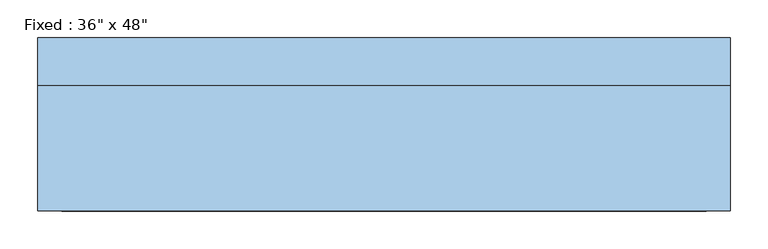
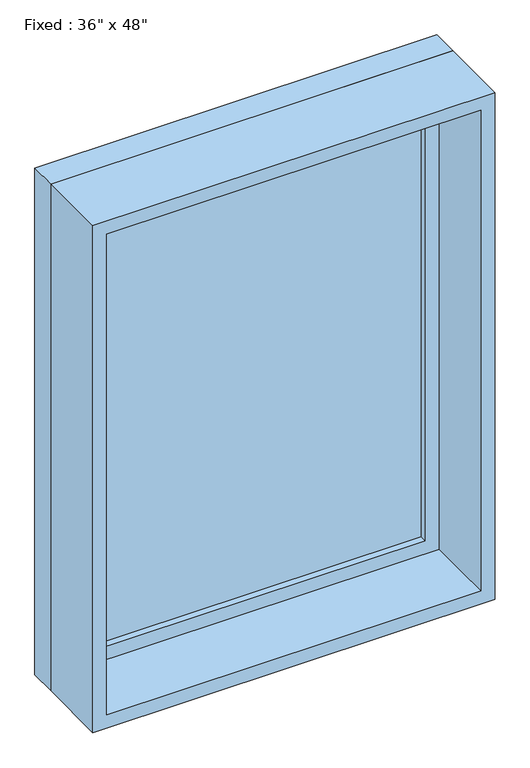
"""IFC4 building model written with IfcOpenShell, lengths in millimetres: window geometry."""

from ifc_helpers import new_model, si_unit, frame, origin, place, context, project, spatial, polyline, outline, extrude, source, transform, mapped, element, save


def window_c1f32544(model_context):
    return source(origin(), model_context, "Body", "SweptSolid", [
        extrude(outline(polyline([(355.6, 66.675), (-431.8, 66.675), (-431.8, 79.375), (355.6, 79.375), (355.6, 66.675)])), frame((0.0, 0.0, 977.9), z_axis=(0.0, 0.0, 1.0), x_axis=(1.0, 0.0, 0.0)), (0.0, 0.0, 1.0), 1092.2),
        extrude(outline(polyline([(2114.55, -476.25), (933.45, -476.25), (933.45, 400.05), (2114.55, 400.05), (2114.55, -476.25)]), holes=[polyline([(2070.1, -431.8), (2070.1, 355.6), (977.9, 355.6), (977.9, -431.8), (2070.1, -431.8)])]), frame((0.0, 50.8, 0.0), z_axis=(0.0, 1.0, 0.0), x_axis=(0.0, 0.0, 1.0)), (0.0, 0.0, 1.0), 44.45),
        extrude(outline(polyline([(2133.6, -495.3), (914.4, -495.3), (914.4, 419.1), (2133.6, 419.1), (2133.6, -495.3)]), holes=[polyline([(2101.85, -463.55), (2101.85, 387.35), (946.15, 387.35), (946.15, -463.55), (2101.85, -463.55)])]), frame((0.0, -114.3, 0.0), z_axis=(0.0, 1.0, 0.0), x_axis=(0.0, 0.0, 1.0)), (0.0, 0.0, 1.0), 165.1),
        extrude(outline(polyline([(2133.6, 419.1), (2133.6, -495.3), (914.4, -495.3), (914.4, 419.1), (2133.6, 419.1)]), holes=[polyline([(2114.55, 400.05), (933.45, 400.05), (933.45, -476.25), (2114.55, -476.25), (2114.55, 400.05)])]), frame((0.0, 50.8, 0.0), z_axis=(0.0, 1.0, 0.0), x_axis=(0.0, 0.0, 1.0)), (0.0, 0.0, 1.0), 63.5),
    ])


if __name__ == "__main__":
    model = new_model("IFC4")
    model_context = context("Model", 3, world=origin())
    ifc_project = project(units=[si_unit("LENGTHUNIT", "METRE", prefix="MILLI")], contexts=[model_context])
    site = spatial("IfcSite", under=ifc_project)
    building = spatial("IfcBuilding", under=site)
    placement = place(None, origin())
    window_shape = window_c1f32544(model_context)
    element("IfcWindow", 1, ObjectType="Fixed : 36\" x 48\"", at=placement, inside=building, context=model_context, shape_type="MappedRepresentation", body=[
        mapped(window_shape, transform((0.0, 0.0, 0.0), x_axis=(1.0, 0.0, 0.0), y_axis=(0.0, 1.0, 0.0), z_axis=(0.0, 0.0, 1.0))),
    ])
    save(model, "model.ifc")

# Revit data of these elements
# Type "Fixed : 36\" x 48\""
#   Type Mark = "1"
#   Construction Type Id = "GSP4R"
#   Assembly Code = "B2020100"
#   Analytic Construction = "1/8 in Pilkington single glazing"
#   Visual Light Transmittance = 0.9
#   Solar Heat Gain Coefficient = 0.78
#   Heat Transfer Coefficient (U) = 0.6496 BTU/(h·ft²·°F)
#   Height = 4' - 0"
#   Default Sill Height = 3' - 0"
#   Width = 3' - 0"
#   Window Inset = 0' - 0 3/4"
#   Define Thermal Properties by = 1
#   Glass Pane Material = Glass
#   Sash Material = Sash
#   Wall Closure = (empty or 0)
# Element 1 (IfcWindow, "Fixed : 36\" x 48\"")
#   Materials on its faces: "Sash", "Glass"
# Materials
#   "Glass": class "Glass", colour RGB 0 128 192, transparency 0.75, Description = "Soda Lime Glass", Cost = 0
#   "Sash": class "Wood", colour RGB 224 178 126, transparency 0
